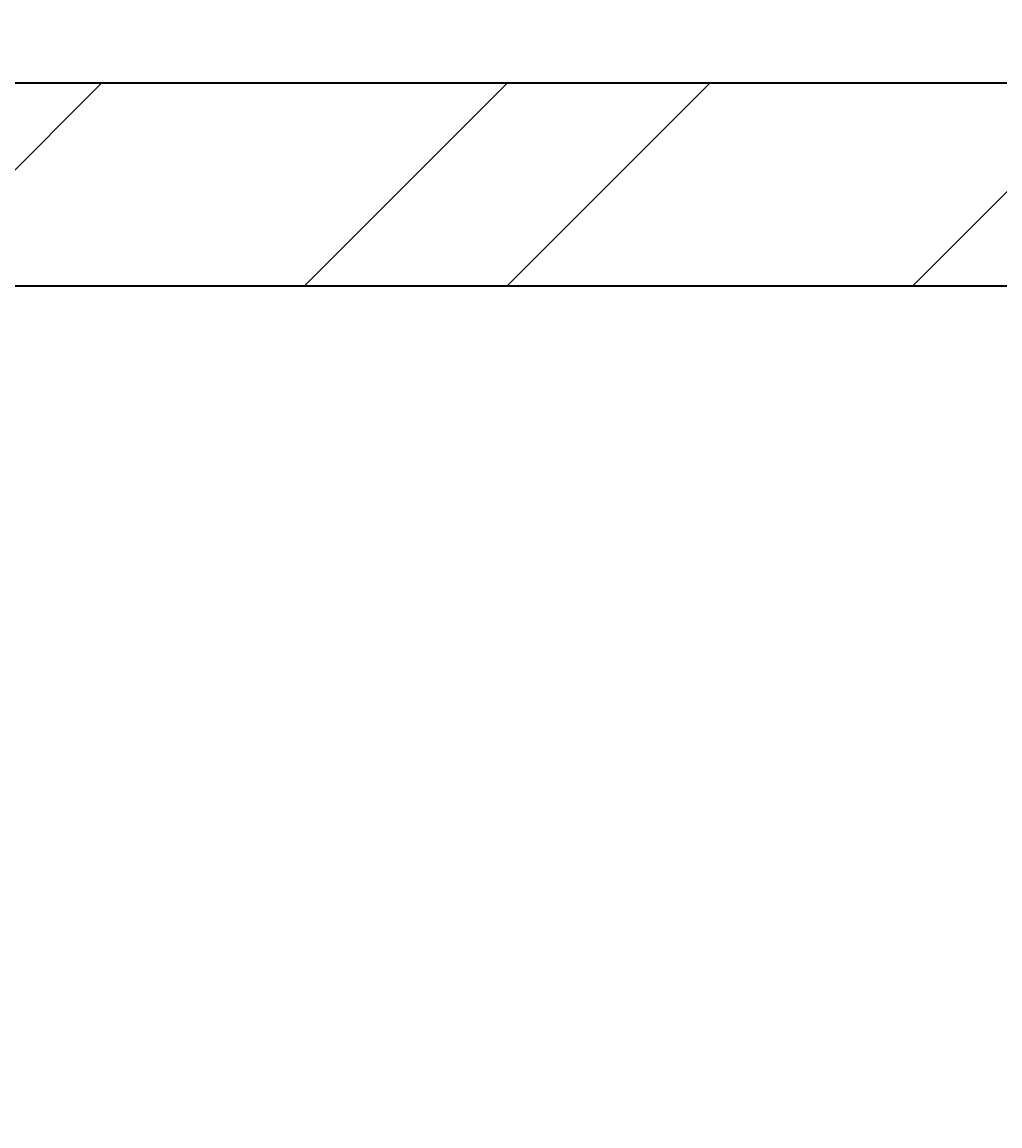
# Model space of a CAD drawing. Units: inches. Extents: x 1962 to 2771, y 1245 to 2660.
# Tile 80 of 114: x 2617.5 to 2639.16, y 2106.74 to 2131.19. Entities that reach past the tile are written whole.
import ezdxf

# ---------------------------------------------------------------- set-up
doc = ezdxf.new("R2010")
doc.units = ezdxf.units.IN
for name, color, linetype, lineweight in [('A-ANNO-DIMS', 2, 'Continuous', 18), ('A-WALL', 7, 'Continuous', 35), ('A-WALL-PATT', 252, 'Continuous', 13)]:
    doc.layers.add(name, color=color, linetype=linetype, lineweight=lineweight)
doc.styles.get("Standard").update_dxf_attribs({"font": 'arial.ttf'})
doc.dimstyles.get("Standard").update_dxf_attribs({"dimtxt": 0.18, "dimasz": 0.18, "dimexe": 0.18, "dimexo": 0.0625, "dimgap": 0.09, "dimtad": 0, "dimtih": 1, "dimtoh": 1, "dimdec": 4, "dimzin": 0, "dimdsep": 46, "dimtxsty": 'Standard', "dimcen": 0.09, "dimadec": 0, "dimazin": 0, "dimtfac": 1, "dimtdec": 4, "dimtofl": 0, "dimtmove": 0, "dimatfit": 3, "dimfxl": 1, "dimtolj": 1, "dimtzin": 0, "dimarcsym": 0})

# ---------------------------------------------------------------- blocks, each defined once
blk = doc.blocks.new('*D40')
at = {"layer": 'A-ANNO-DIMS', "color": 0, "lineweight": -2, "transparency": 16777216}
for p, q in [((2072.02, 2033.906), (2072.02, 2583.474)), ((2660.807, 2524.406), (2660.807, 2583.474)), ((2072.2, 2583.294), (2366.02, 2583.294)), ((2660.627, 2583.294), (2366.808, 2583.294))]:
    blk.add_line(p, q, dxfattribs=at)
at = {"layer": 'A-ANNO-DIMS', "color": 0, "transparency": 16777216}
for points in [[(2072.2, 2583.324), (2072.2, 2583.264), (2072.02, 2583.294)], [(2660.627, 2583.324), (2660.627, 2583.264), (2660.807, 2583.294)]]:
    blk.add_solid(points, dxfattribs=at)
at = {"layer": 'Defpoints', "color": 0, "transparency": 16777216}
for p in [(2660.807, 2583.294), (2660.807, 2524.344), (2072.02, 2033.844)]:
    blk.add_point(p, dxfattribs=at)
at = {"layer": 'A-ANNO-DIMS', "color": 0, "transparency": 16777216, "insert": (2366.414, 2583.294), "char_height": 0.18, "attachment_point": 5}
blk.add_mtext('\\A1;588.8', dxfattribs=at)

msp = doc.modelspace()

# ---------------------------------------------------------------- hatches: boundary and pattern name
at = {"layer": 'A-WALL-PATT'}
h = msp.add_hatch(dxfattribs=at)
h.set_pattern_fill('ANSI32', color=256)
h.paths.add_polyline_path([(2090.8074, 2467.3437), (2141.6481, 2467.3437), (2141.6481, 2469.5937), (2141.6481, 2471.8437), (2086.3074, 2471.8437), (2086.3074, 2422.5333), (2090.8074, 2422.5333)])
h.paths.add_polyline_path([(2282.7664, 2471.8437), (2204.8982, 2471.8437), (2204.8982, 2467.3437), (2234.8074, 2467.3437), (2234.8074, 2311.3437), (2228.7492, 2311.3437), (2228.7492, 2306.8437), (2234.8074, 2306.8437), (2331.9227, 2306.8437), (2331.9227, 2309.0937), (2331.9227, 2311.3437), (2239.3074, 2311.3437), (2239.3074, 2467.3437), (2282.7664, 2467.3437), (2282.7664, 2469.5937)])
h.paths.add_polyline_path([(2471.4531, 2519.8437), (2552.011, 2519.8437), (2564.3996, 2519.8437), (2564.3996, 2511.1389), (2568.8996, 2511.1389), (2568.8996, 2524.3437), (2466.9531, 2524.3437), (2466.9531, 2471.8437), (2450.0749, 2471.8437), (2446.4672, 2471.8437), (2446.4672, 2467.3437), (2450.0749, 2467.3437), (2475.9988, 2467.3437), (2475.9988, 2469.5937), (2475.9988, 2471.8437), (2471.4531, 2471.8437)])
h.paths.add_polyline_path([(2575.2231, 2469.5937), (2575.2231, 2471.8437), (2568.8996, 2471.8437), (2568.8996, 2487.1389), (2564.3996, 2487.1389), (2564.3996, 2471.8437), (2556.511, 2471.8437), (2499.2904, 2471.8437), (2499.2904, 2467.3437), (2507.8074, 2467.3437), (2507.8074, 2311.3437), (2414.863, 2311.3437), (2414.863, 2306.8437), (2512.3074, 2306.8437), (2517.0114, 2306.8437), (2517.0114, 2309.0937), (2517.0114, 2311.3437), (2512.3074, 2311.3437), (2512.3074, 2467.3437), (2575.2231, 2467.3437)])
h.paths.add_polyline_path([(2660.8074, 2471.8437), (2600.9602, 2471.8437), (2600.9602, 2467.3437), (2656.3074, 2467.3437), (2656.3074, 2432.5704), (2660.8074, 2432.5704)])
h.paths.add_polyline_path([(2660.8074, 2372.5704), (2656.3074, 2372.5704), (2656.3074, 2311.3437), (2600.276, 2311.3437), (2600.276, 2309.0937), (2600.276, 2306.8437), (2656.3074, 2306.8437), (2656.3074, 2296.2593), (2660.8074, 2296.2593)])
h.paths.add_polyline_path([(2572.3074, 2306.8437), (2577.1385, 2306.8437), (2577.1385, 2311.3437), (2551.082, 2311.3437), (2551.082, 2306.8437), (2567.8074, 2306.8437), (2567.8074, 2258.8437), (2540.0574, 2258.8437), (2540.0574, 2256.5937), (2540.0574, 2254.3437), (2567.8074, 2254.3437), (2656.3074, 2254.3437), (2656.3074, 2236.9085), (2660.8074, 2236.9085), (2660.8074, 2272.2593), (2656.3074, 2272.2593), (2656.3074, 2258.8437), (2572.3074, 2258.8437)])
h.paths.add_polyline_path([(2512.3074, 2254.3437), (2518.8716, 2254.3437), (2518.8716, 2256.5937), (2518.8716, 2258.8437), (2507.8074, 2258.8437), (2507.8074, 2177.8437), (2567.8074, 2177.8437), (2567.8074, 2172.9628), (2572.3074, 2172.9628), (2572.3074, 2177.8437), (2656.3074, 2177.8437), (2656.3074, 2166.4846), (2660.8074, 2166.4846), (2660.8074, 2200.9085), (2656.3074, 2200.9085), (2656.3074, 2182.3437), (2512.3074, 2182.3437)])
h.paths.add_polyline_path([(2656.3074, 2129.8437), (2572.3074, 2129.8437), (2572.3074, 2150.3044), (2570.0574, 2150.3044), (2567.8074, 2150.3044), (2567.8074, 2129.8437), (2507.8074, 2129.8437), (2507.8074, 2116.3027), (2510.0574, 2116.3027), (2512.3074, 2116.3027), (2512.3074, 2125.3437), (2567.8074, 2125.3437), (2572.3074, 2125.3437), (2656.3074, 2125.3437)])
h.paths.add_polyline_path([(2090.8074, 2362.5333), (2086.3074, 2362.5333), (2086.3074, 2298.6242), (2090.8074, 2298.6242), (2090.8074, 2306.8437), (2174.8074, 2306.8437), (2174.8074, 2286.4178), (2179.3074, 2286.4178), (2179.3074, 2306.8437), (2192.8641, 2306.8437), (2192.8641, 2309.0937), (2192.8641, 2311.3437), (2090.8074, 2311.3437)])
h.paths.add_polyline_path([(2209.156, 2258.8437), (2179.3074, 2258.8437), (2179.3074, 2263.2236), (2177.0574, 2263.2236), (2174.8074, 2263.2236), (2174.8074, 2258.8437), (2090.8074, 2258.8437), (2090.8074, 2274.6242), (2086.3074, 2274.6242), (2086.3074, 2238.2967), (2088.5574, 2238.2967), (2090.8074, 2238.2967), (2090.8074, 2254.3437), (2209.156, 2254.3437)])
h.paths.add_polyline_path([(2090.8074, 2177.8437), (2234.8074, 2177.8437), (2234.8074, 2173.1428), (2239.3074, 2173.1428), (2239.3074, 2258.8437), (2230.8442, 2258.8437), (2230.8442, 2256.5937), (2230.8442, 2254.3437), (2234.8074, 2254.3437), (2234.8074, 2182.3437), (2090.8074, 2182.3437), (2090.8074, 2202.2967), (2086.3074, 2202.2967), (2086.3074, 2140.0389), (2090.8074, 2140.0389)])
h.paths.add_polyline_path([(2090.8074, 2080.0389), (2086.3074, 2080.0389), (2086.3074, 2033.8437), (2090.8074, 2033.8437)], flags=17)
h.paths.add_polyline_path([(2244.9405, 2033.8437), (2239.3074, 2033.8437), (2239.3074, 2142.0665), (2237.2592, 2142.0665), (2234.8074, 2142.0665), (2234.8074, 2033.8437), (2090.8074, 2033.8437), (2076.5204, 2033.8437), (2072.0204, 2033.8437), (2072.0204, 2000.4493), (2076.5204, 2000.4493), (2076.5204, 2029.3437), (2090.8074, 2029.3437), (2244.9405, 2029.3437), (2244.9405, 2031.5937)])
h.paths.add_polyline_path([(2234.8074, 1933.3437), (2076.5204, 1933.3437), (2076.5204, 1952.4493), (2074.2704, 1952.4493), (2072.0204, 1952.4493), (2072.0204, 1933.3437), (2072.0204, 1928.8437), (2234.8074, 1928.8437)])
h.paths.add_polyline_path([(2090.8074, 1928.8437), (2086.3074, 1928.8437), (2086.3074, 1906.5013), (2090.8074, 1906.5013)])
h.paths.add_polyline_path([(2090.8074, 1846.5013), (2086.3074, 1846.5013), (2086.3074, 1769.9917), (2088.5574, 1769.9917), (2090.8074, 1769.9917), (2090.8074, 1780.3437), (2234.8074, 1780.3437), (2234.8074, 1708.3437), (2230.3764, 1708.3437), (2230.3764, 1703.8437), (2239.3074, 1703.8437), (2239.3074, 1792.6669), (2237.0574, 1792.6669), (2234.8074, 1792.6669), (2234.8074, 1784.8437), (2090.8074, 1784.8437)])
h.paths.add_polyline_path([(2239.3074, 1928.8437), (2244.9405, 1928.8437), (2244.9405, 1931.0937), (2244.9405, 1933.3437), (2234.8074, 1933.3437), (2234.8074, 1928.8437), (2234.8074, 1825.5949), (2239.3074, 1825.5949)])
h.paths.add_polyline_path([(2148.0425, 1649.0937), (2148.0425, 1651.3437), (2090.8074, 1651.3437), (2090.8074, 1646.8437), (2148.0425, 1646.8437)], flags=0)
h.paths.add_polyline_path([(2207.5601, 1708.3437), (2090.8074, 1708.3437), (2090.8074, 1703.8437), (2174.8074, 1703.8437), (2174.8074, 1651.3437), (2170.4457, 1651.3437), (2170.4457, 1646.8437), (2195.9924, 1646.8437), (2195.9924, 1649.0937), (2195.9924, 1651.3437), (2179.3074, 1651.3437), (2179.3074, 1703.8437), (2207.5601, 1703.8437), (2207.5601, 1706.0937)])
h.paths.add_polyline_path([(2090.8074, 1733.9917), (2086.3074, 1733.9917), (2086.3074, 1696.1032), (2088.5574, 1696.1032), (2090.8074, 1696.1032)])
h.paths.add_polyline_path([(2090.8074, 1672.1032), (2086.3074, 1672.1032), (2086.3074, 1600.3335), (2090.8074, 1600.3335)])
h.paths.add_polyline_path([(2090.8074, 1540.3335), (2086.3074, 1540.3335), (2086.3074, 1486.3437), (2139.6766, 1486.3437), (2139.6766, 1490.8437), (2090.8074, 1490.8437)])
h.paths.add_polyline_path([(2302.3876, 1490.8437), (2239.3074, 1490.8437), (2239.3074, 1646.8437), (2335.9994, 1646.8437), (2335.9994, 1651.3437), (2229.884, 1651.3437), (2229.884, 1646.8437), (2234.8074, 1646.8437), (2234.8074, 1490.8437), (2202.7103, 1490.8437), (2202.7103, 1488.5937), (2202.7103, 1486.3437), (2275.0699, 1486.3437), (2275.0699, 1475.772), (2279.5699, 1475.772), (2279.5699, 1486.3437), (2302.3876, 1486.3437)])
h.paths.add_polyline_path([(2279.5699, 1451.772), (2275.0699, 1451.772), (2275.0699, 1438.3437), (2174.8074, 1438.3437), (2174.8074, 1486.3437), (2179.7922, 1486.3437), (2179.7922, 1490.8437), (2163.3585, 1490.8437), (2163.3585, 1488.5937), (2163.3585, 1486.3437), (2170.3074, 1486.3437), (2170.3074, 1433.8437), (2279.5699, 1433.8437)])
h.paths.add_polyline_path([(2427.2363, 1490.8437), (2375.8074, 1490.8437), (2375.8074, 1646.8437), (2381.6401, 1646.8437), (2381.6401, 1651.3437), (2365.887, 1651.3437), (2365.887, 1649.0937), (2365.887, 1646.8437), (2371.3074, 1646.8437), (2371.3074, 1490.8437), (2327.5627, 1490.8437), (2327.5627, 1488.5937), (2327.5627, 1486.3437), (2371.3074, 1486.3437), (2371.3074, 1433.8437), (2375.8074, 1433.8437), (2375.8074, 1486.3437), (2427.2363, 1486.3437)])
h.paths.add_polyline_path([(2512.3074, 1646.8437), (2519.4351, 1646.8437), (2519.4351, 1649.0937), (2519.4351, 1651.3437), (2507.8074, 1651.3437), (2416.0063, 1651.3437), (2416.0063, 1649.0937), (2416.0063, 1646.8437), (2507.8074, 1646.8437), (2507.8074, 1490.8437), (2497.0532, 1490.8437), (2497.0532, 1488.5937), (2497.0532, 1486.3437), (2574.9344, 1486.3437), (2574.9344, 1476.0181), (2579.4344, 1476.0181), (2579.4344, 1486.3437), (2584.4872, 1486.3437), (2584.3074, 1490.8437), (2512.3074, 1490.8437)])
h.paths.add_polyline_path([(2470.5091, 1486.3437), (2473.9767, 1486.3437), (2473.9767, 1490.8437), (2449.6605, 1490.8437), (2449.6605, 1488.5937), (2449.6605, 1486.3437), (2466.0091, 1486.3437), (2466.0091, 1433.8437), (2470.5091, 1433.8437), (2579.4344, 1433.8437), (2579.4344, 1452.0181), (2574.9344, 1452.0181), (2574.9344, 1438.3437), (2554.5091, 1438.3437), (2470.5091, 1438.3437)])
h.paths.add_polyline_path([(2656.3074, 1490.8437), (2611.86, 1490.8437), (2611.86, 1486.3437), (2656.3074, 1486.3437)])
h.paths.add_polyline_path([(2660.8074, 1532.7007), (2658.5574, 1532.7007), (2656.3074, 1532.7007), (2656.3074, 1486.3437), (2660.8074, 1486.3437)])
h.paths.add_polyline_path([(2660.8074, 1664.9663), (2656.3074, 1664.9663), (2656.3074, 1651.3437), (2602.2313, 1651.3437), (2602.2313, 1646.8437), (2656.3074, 1646.8437), (2656.3074, 1592.7007), (2660.8074, 1592.7007)])
h.paths.add_polyline_path([(2660.8074, 1724.5221), (2656.3074, 1724.5221), (2656.3074, 1703.8437), (2542.4725, 1703.8437), (2542.4725, 1699.3437), (2567.8074, 1699.3437), (2567.8074, 1651.3437), (2552.7766, 1651.3437), (2552.7766, 1649.0937), (2552.7766, 1646.8437), (2577.2878, 1646.8437), (2577.2878, 1649.0937), (2577.2878, 1651.3437), (2572.3074, 1651.3437), (2572.3074, 1699.3437), (2656.3074, 1699.3437), (2656.3074, 1688.9663), (2660.8074, 1688.9663)])
h.paths.add_polyline_path([(2660.8074, 1880.6524), (2656.3074, 1880.6524), (2656.3074, 1832.8437), (2512.3074, 1832.8437), (2512.3074, 1837.8959), (2507.8074, 1837.8959), (2507.8074, 1828.3437), (2567.8074, 1828.3437), (2567.8074, 1804.3437), (2572.3074, 1804.3437), (2572.3074, 1828.3437), (2656.3074, 1828.3437), (2656.3074, 1818.6778), (2660.8074, 1818.6778)])
h.paths.add_polyline_path([(2660.8074, 1794.6778), (2656.3074, 1794.6778), (2656.3074, 1780.3437), (2572.3074, 1780.3437), (2572.3074, 1783.0303), (2570.0574, 1783.0303), (2567.8074, 1783.0303), (2567.8074, 1780.3437), (2507.8074, 1780.3437), (2507.8074, 1699.3437), (2517.8858, 1699.3437), (2517.8858, 1701.5937), (2517.8858, 1703.8437), (2512.3074, 1703.8437), (2512.3074, 1775.8437), (2656.3074, 1775.8437), (2656.3074, 1760.5221), (2660.8074, 1760.5221)])
h.paths.add_polyline_path([(2660.8074, 1981.3437), (2660.8074, 2020.2808), (2658.5574, 2020.2808), (2656.3074, 2020.2808), (2656.3074, 1981.3437), (2512.3074, 1981.3437), (2512.3074, 2086.6996), (2507.8074, 2086.6996), (2507.8074, 1981.3437), (2375.8074, 1981.3437), (2375.8074, 1986.8505), (2373.5574, 1986.8505), (2371.3074, 1986.8505), (2371.3074, 1973.2607), (2375.8074, 1973.2607), (2375.8074, 1976.8437), (2507.8074, 1976.8437), (2507.8074, 1865.4281), (2510.0574, 1865.4281), (2512.3074, 1865.4281), (2512.3074, 1976.8437), (2660.8074, 1976.8437)])
h.paths.add_polyline_path([(2375.8074, 1940.297), (2373.5574, 1940.297), (2371.3074, 1940.297), (2371.3074, 1933.3437), (2278.4434, 1933.3437), (2278.4434, 1928.8437), (2371.3074, 1928.8437), (2371.3074, 1651.3437), (2375.8074, 1651.3437)])
h.paths.add_polyline_path([(2660.8074, 1976.8437), (2656.3074, 1976.8437), (2656.3074, 1940.6524), (2660.8074, 1940.6524)], flags=17)
h.paths.add_polyline_path([(2660.8074, 2142.4846), (2656.3074, 2142.4846), (2656.3074, 2080.2808), (2660.8074, 2080.2808)])
h.paths.add_polyline_path([(2381.4189, 2311.3437), (2375.8074, 2311.3437), (2375.8074, 2467.3437), (2424.7242, 2467.3437), (2424.7242, 2469.5937), (2424.7242, 2471.8437), (2375.8074, 2471.8437), (2375.8074, 2524.3437), (2371.3074, 2524.3437), (2371.3074, 2471.8437), (2307.2097, 2471.8437), (2307.2097, 2467.3437), (2371.3074, 2467.3437), (2371.3074, 2311.3437), (2366.8901, 2311.3437), (2366.8901, 2306.8437), (2371.3074, 2306.8437), (2371.3074, 2033.8437), (2279.6589, 2033.8437), (2279.6589, 2029.3437), (2371.3074, 2029.3437), (2371.3074, 2014.2598), (2375.8074, 2014.2598), (2375.8074, 2306.8437), (2381.4189, 2306.8437)])
h.paths.add_polyline_path([(2263.3074, 2524.3437), (2170.3074, 2524.3437), (2170.3074, 2519.8437), (2170.3074, 2471.8437), (2165.0312, 2471.8437), (2165.0312, 2467.3437), (2179.6721, 2467.3437), (2179.6721, 2469.5161), (2179.6721, 2471.8437), (2174.8074, 2471.8437), (2174.8074, 2519.8437), (2258.8074, 2519.8437), (2258.8074, 2511.6436), (2263.3074, 2511.6436)])
h.paths.add_polyline_path([(2245.0232, 1361.4123), (2492.9468, 1361.4123), (2492.9468, 1398.505), (2245.0232, 1398.505)], flags=9)
h.paths.add_polyline_path([(2388.1434, 2086.6936), (2425.0704, 2086.6936), (2425.0704, 2105.3509), (2388.1434, 2105.3509)], flags=9)
h.paths.add_polyline_path([(2404.922, 2242.6744), (2445.7337, 2242.6744), (2445.7337, 2261.3318), (2404.922, 2261.3318)], flags=9)
h.paths.add_polyline_path([(2269.4107, 2156.7935), (2306.3378, 2156.7935), (2306.3378, 2175.4508), (2269.4107, 2175.4508)], flags=9)
h.paths.add_polyline_path([(2269.3277, 2233.4343), (2306.2547, 2233.4343), (2306.2547, 2252.0917), (2269.3277, 2252.0917)], flags=9)
h.paths.add_polyline_path([(2431.6052, 2320.6922), (2470.4456, 2320.6922), (2470.4456, 2339.3495), (2431.6052, 2339.3495)], flags=25)
h.paths.add_polyline_path([(2249.6902, 2315.7608), (2288.5306, 2315.7608), (2288.5306, 2334.4182), (2249.6902, 2334.4182)], flags=25)
h.paths.add_polyline_path([(2096.9301, 2314.3181), (2135.7704, 2314.3181), (2135.7704, 2332.9755), (2096.9301, 2332.9755)], flags=25)
h.paths.add_polyline_path([(2134.3475, 2285.7089), (2161.4655, 2285.7089), (2161.4655, 2304.3662), (2134.3475, 2304.3662)], flags=9)
h.paths.add_polyline_path([(2126.5155, 2209.4076), (2159.9227, 2209.4076), (2159.9227, 2228.065), (2126.5155, 2228.065)], flags=25)
h.paths.add_polyline_path([(2110.5753, 2141.5299), (2149.4157, 2141.5299), (2149.4157, 2160.1872), (2110.5753, 2160.1872)], flags=25)
h.paths.add_polyline_path([(2249.8618, 1968.3317), (2286.3966, 1968.3317), (2286.3966, 1986.989), (2249.8618, 1986.989)], flags=9)
h.paths.add_polyline_path([(2395.9507, 1777.0051), (2436.7624, 1777.0051), (2436.7624, 1795.6625), (2395.9507, 1795.6625)], flags=9)
h.paths.add_polyline_path([(2398.5259, 1888.5651), (2435.0062, 1888.5651), (2435.0062, 1907.2224), (2398.5259, 1907.2224)], flags=25)
h.paths.add_polyline_path([(2259.3506, 1728.3559), (2296.2776, 1728.3559), (2296.2776, 1747.0132), (2259.3506, 1747.0132)], flags=9)
h.paths.add_polyline_path([(2271.3698, 1845.268), (2308.2968, 1845.268), (2308.2968, 1863.9253), (2271.3698, 1863.9253)], flags=9)
h.paths.add_polyline_path([(2120.9355, 1786.3027), (2159.7759, 1786.3027), (2159.7759, 1804.9601), (2120.9355, 1804.9601)], flags=25)
h.paths.add_polyline_path([(2121.3164, 1732.1043), (2154.7236, 1732.1043), (2154.7236, 1750.7616), (2121.3164, 1750.7616)], flags=25)
h.paths.add_polyline_path([(2118.3706, 1678.8997), (2147.5282, 1678.8997), (2147.5282, 1697.557), (2118.3706, 1697.557)], flags=25)
h.paths.add_polyline_path([(2385.9227, 1493.557), (2424.763, 1493.557), (2424.763, 1512.2143), (2385.9227, 1512.2143)], flags=25)
h.paths.add_polyline_path([(2248.7058, 1500.0256), (2287.5462, 1500.0256), (2287.5462, 1518.6829), (2248.7058, 1518.6829)], flags=25)
h.paths.add_polyline_path([(2104.1669, 1617.3771), (2143.0073, 1617.3771), (2143.0073, 1636.0344), (2104.1669, 1636.0344)], flags=9)
h.paths.add_polyline_path([(2096.0714, 1447.8824), (2137.3845, 1447.8824), (2137.3845, 1458.1859), (2096.0714, 1458.1859)], flags=9)
h.paths.add_polyline_path([(2180.6114, 1440.325), (2209.7689, 1440.325), (2209.7689, 1458.9823), (2180.6114, 1458.9823)], flags=25)
h.paths.add_polyline_path([(2316.1698, 1447.9637), (2357.4829, 1447.9637), (2357.4829, 1458.2673), (2316.1698, 1458.2673)], flags=9)
h.paths.add_polyline_path([(2397.6187, 1447.9637), (2438.9318, 1447.9637), (2438.9318, 1458.2673), (2397.6187, 1458.2673)], flags=9)
h.paths.add_polyline_path([(2473.0778, 1439.5953), (2502.2354, 1439.5953), (2502.2354, 1458.2527), (2473.0778, 1458.2527)], flags=25)
h.paths.add_polyline_path([(2589.7027, 1447.8819), (2631.0158, 1447.8819), (2631.0158, 1458.1855), (2589.7027, 1458.1855)], flags=9)
h.paths.add_polyline_path([(2522.4009, 1497.5285), (2561.2413, 1497.5285), (2561.2413, 1516.1859), (2522.4009, 1516.1859)], flags=25)
h.paths.add_polyline_path([(2579.6565, 1671.3482), (2608.8141, 1671.3482), (2608.8141, 1690.0056), (2579.6565, 1690.0056)], flags=25)
h.paths.add_polyline_path([(2544.7038, 1725.5064), (2578.1111, 1725.5064), (2578.1111, 1744.1637), (2544.7038, 1744.1637)], flags=25)
h.paths.add_polyline_path([(2578.1191, 1807.472), (2607.2766, 1807.472), (2607.2766, 1826.1293), (2578.1191, 1826.1293)], flags=25)
h.paths.add_polyline_path([(2595.0614, 1835.1839), (2633.9018, 1835.1839), (2633.9018, 1853.8413), (2595.0614, 1853.8413)], flags=25)
h.paths.add_polyline_path([(2567.0097, 2097.7035), (2605.8501, 2097.7035), (2605.8501, 2116.3609), (2567.0097, 2116.3609)], flags=9)
h.paths.add_polyline_path([(2586.644, 2134.6454), (2615.8015, 2134.6454), (2615.8015, 2153.3027), (2586.644, 2153.3027)], flags=9)
h.paths.add_polyline_path([(2544.6185, 2212.6783), (2578.0258, 2212.6783), (2578.0258, 2231.3356), (2544.6185, 2231.3356)], flags=25)
h.paths.add_polyline_path([(2577.0273, 2256.9023), (2606.1849, 2256.9023), (2606.1849, 2275.5597), (2577.0273, 2275.5597)], flags=24)
h.paths.add_polyline_path([(2605.2683, 2315.2821), (2644.1087, 2315.2821), (2644.1087, 2333.9395), (2605.2683, 2333.9395)], flags=25)
h.paths.add_polyline_path([(2583.1244, 2496.1815), (2624.4375, 2496.1815), (2624.4375, 2506.4851), (2583.1244, 2506.4851)], flags=9)
h.paths.add_polyline_path([(2474.761, 2497.0823), (2503.9185, 2497.0823), (2503.9185, 2515.7397), (2474.761, 2515.7397)], flags=25)
h.paths.add_polyline_path([(2387.5787, 2494.2563), (2428.902, 2494.2563), (2428.902, 2504.5598), (2387.5787, 2504.5598)], flags=9)
h.paths.add_polyline_path([(2300.1657, 2500.1564), (2341.4788, 2500.1564), (2341.4788, 2510.46), (2300.1657, 2510.46)], flags=25)
h.paths.add_polyline_path([(2176.8589, 2497.5843), (2206.0165, 2497.5843), (2206.0165, 2516.2416), (2176.8589, 2516.2416)], flags=25)
h.paths.add_polyline_path([(2097.4668, 2494.9762), (2138.7799, 2494.9762), (2138.7799, 2505.2798), (2097.4668, 2505.2798)], flags=9)

# ---------------------------------------------------------------- linework, layer by layer
at = {"layer": 'A-WALL'}
for p, q in [((2572.3074, 2129.8437), (2656.3074, 2129.8437)), ((2656.3074, 2125.3437), (2572.3074, 2125.3437))]:
    msp.add_line(p, q, dxfattribs=at)

# ---------------------------------------------------------------- dimensions: what is measured, and where the dimension line sits
at = {"layer": 'A-ANNO-DIMS'}
dim = msp.add_linear_dim(base=(2660.8074, 2583.2937), p1=(2072.0204, 2033.8437), p2=(2660.8074, 2524.3437), dimstyle='Standard', override={"dimdec": 1, "dimlfac": 1, "dimrnd": 0, "dimzin": 0, "dimdsep": 46, "dimlunit": 2}, dxfattribs=at)
dim.commit()
dim.dimension.update_dxf_attribs({"geometry": '*D40', "text_midpoint": (2366.4139, 2583.2937)})

doc.saveas('drawing.dxf')
